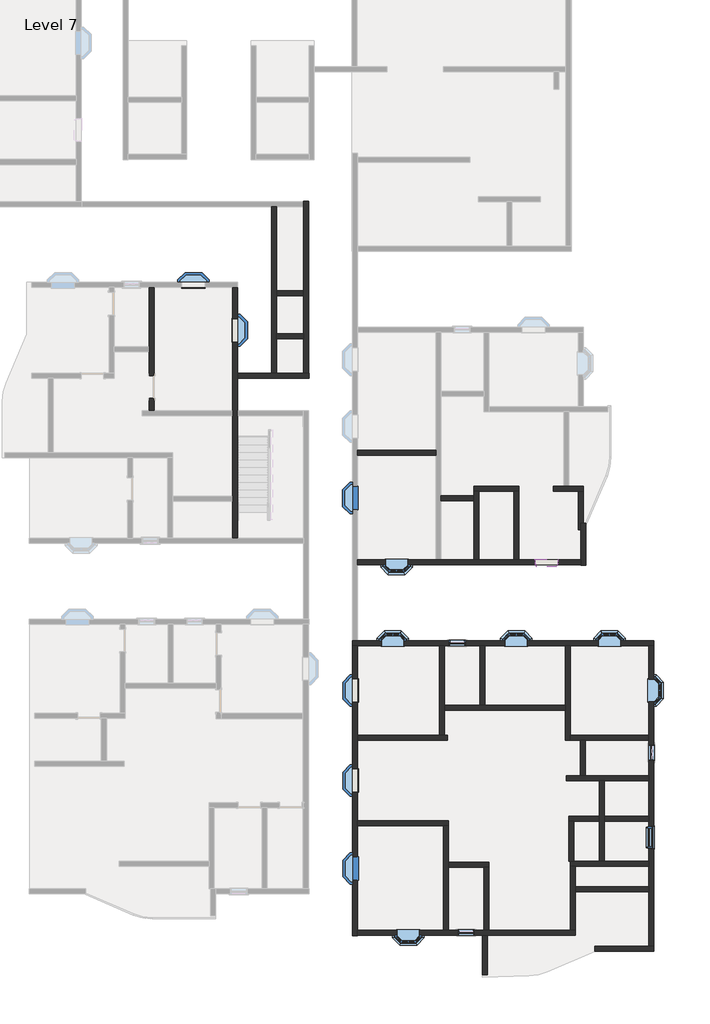
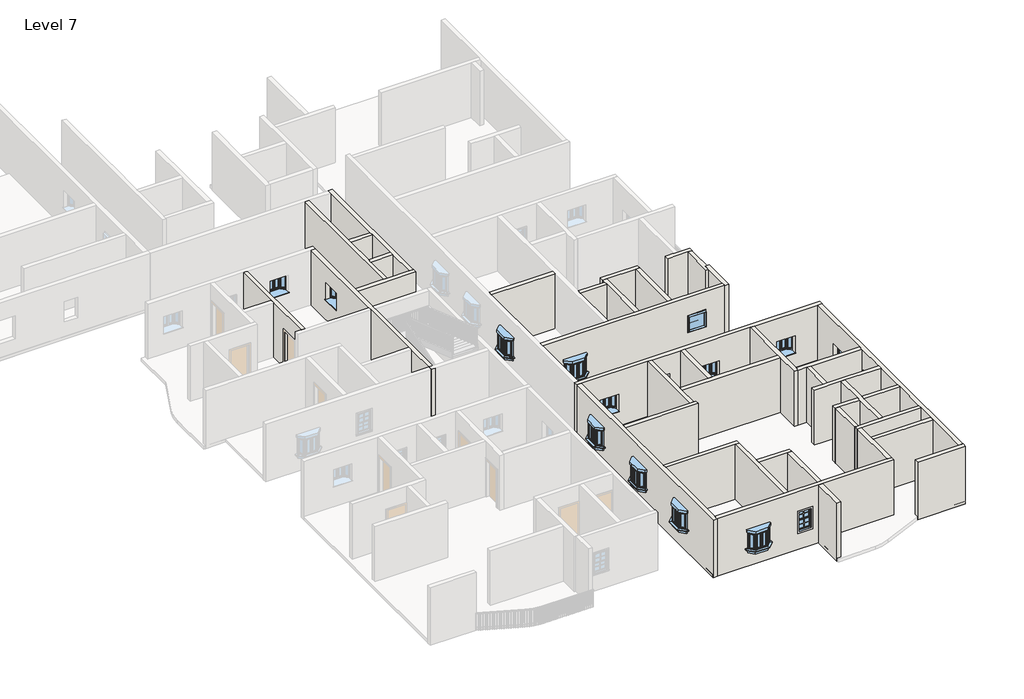
# One storey, part 2 of 14: 40 walls, 17 windows.
"""IFC4 building model written with IfcOpenShell, lengths in millimetres."""

from ifc_helpers import new_model, si_unit, frame, origin, place, context, project, spatial, polyline, outline, extrude, faceted_brep, transform, mapped, element, save
from components import window_910x910mm_67ef725a, window_8debb0fa, windows_sgl_w_glazing_bars_910x910mm_256712d0

model = new_model("IFC4")

# Units and contexts
model_context = context("Model", 3, world=origin())
ifc_project = project(units=[si_unit("LENGTHUNIT", "METRE", prefix="MILLI")], contexts=[model_context])

# Site, building, storey
site = spatial("IfcSite", under=ifc_project)
building = spatial("IfcBuilding", under=site)
storey = spatial("IfcBuildingStorey", under=building, Name="Level 7", Elevation=18288.0)

# Walls
placement = place(None, origin())
element("IfcWall", 1, ObjectType="4.5\" p", at=placement, inside=storey, context=model_context, shape_type="SweptSolid", body=[
    extrude(outline(polyline([(6070.4380523, -28382.7374148), (6070.4380523, -26796.6042694), (6273.6380523, -26796.6042694), (6273.6380523, -28382.7374148), (6070.4380523, -28382.7374148)])), frame((0.0, 0.0, 18288.0), z_axis=(0.0, 0.0, 1.0), x_axis=(1.0, 0.0, 0.0)), (0.0, 0.0, 1.0), 3048.0),
])
element("IfcWall", 2, ObjectType="4.5\" p", at=placement, inside=storey, context=model_context, shape_type="Brep", body=[
    faceted_brep([(10639.6896214, -27431.6042694, 18288.0), (13030.0380523, -27431.6042694, 18288.0), (13030.0380523, -27431.6042694, 21336.0), (10639.6896214, -27431.6042694, 21336.0), (10639.6896214, -27228.4042694, 18288.0), (10639.6896214, -27228.4042694, 21336.0), (12814.1380523, -27228.4042694, 21336.0), (13017.3380523, -27228.4042694, 21336.0), (13030.0380523, -27228.4042694, 21336.0), (13030.0380523, -27228.4042694, 18288.0), (13017.3380523, -27228.4042694, 18288.0), (12814.1380523, -27228.4042694, 18288.0)], [[[0, 1, 2, 3]], [[4, 5, 6, 7, 8, 9, 10, 11]], [[1, 0, 4, 11, 10, 9]], [[2, 1, 9, 8]], [[3, 2, 8, 7, 6, 5]], [[0, 3, 5, 4]]]),
])
element("IfcWall", 3, ObjectType="4.5\" p", at=placement, inside=storey, context=model_context, shape_type="Brep", body=[
    faceted_brep([(1015.8380523, -18878.1542694, 18288.0), (4648.0380523, -18878.1542694, 18288.0), (4648.0380523, -18878.1542694, 21336.0), (1015.8380523, -18878.1542694, 21336.0), (1015.8380523, -18674.9542694, 18288.0), (1015.8380523, -18674.9542694, 21336.0), (4336.8880523, -18674.9542694, 21336.0), (4540.0880523, -18674.9542694, 21336.0), (4648.0380523, -18674.9542694, 21336.0), (4648.0380523, -18674.9542694, 18288.0), (4540.0880523, -18674.9542694, 18288.0), (4336.8880523, -18674.9542694, 18288.0)], [[[0, 1, 2, 3]], [[4, 5, 6, 7, 8, 9, 10, 11]], [[1, 0, 4, 11, 10, 9]], [[2, 1, 9, 8]], [[3, 2, 8, 7, 6, 5]], [[0, 3, 5, 4]]]),
])
element("IfcWall", 4, ObjectType="4.5\" p", at=placement, inside=storey, context=model_context, shape_type="Brep", body=[
    faceted_brep([(4336.8880523, -15049.1042694, 18288.0), (4336.8880523, -18674.9542694, 18288.0), (4336.8880523, -18674.9542694, 21336.0), (4336.8880523, -15049.1042694, 21336.0), (4540.0880523, -15049.1042694, 18288.0), (4540.0880523, -15049.1042694, 21336.0), (4540.0880523, -17455.7542694, 21336.0), (4540.0880523, -17658.9542694, 21336.0), (4540.0880523, -18674.9542694, 21336.0), (4540.0880523, -18674.9542694, 18288.0), (4540.0880523, -17658.9542694, 18288.0), (4540.0880523, -17455.7542694, 18288.0)], [[[0, 1, 2, 3]], [[4, 5, 6, 7, 8, 9, 10, 11]], [[1, 0, 4, 11, 10, 9]], [[3, 2, 8, 7, 6, 5]], [[0, 3, 5, 4]], [[2, 1, 9, 8]]]),
])
element("IfcWall", 5, ObjectType="4.5\" p", at=placement, inside=storey, context=model_context, shape_type="Brep", body=[
    faceted_brep([(4540.0880523, -17658.9542694, 18288.0), (9442.2880523, -17658.9542694, 18288.0), (9442.2880523, -17658.9542694, 21336.0), (4540.0880523, -17658.9542694, 21336.0), (4540.0880523, -17455.7542694, 18288.0), (4540.0880523, -17455.7542694, 21336.0), (5975.1880523, -17455.7542694, 21336.0), (6178.3880523, -17455.7542694, 21336.0), (9442.2880523, -17455.7542694, 21336.0), (9442.2880523, -17455.7542694, 18288.0), (6178.3880523, -17455.7542694, 18288.0), (5975.1880523, -17455.7542694, 18288.0)], [[[0, 1, 2, 3]], [[4, 5, 6, 7, 8, 9, 10, 11]], [[1, 0, 4, 11, 10, 9]], [[3, 2, 8, 7, 6, 5]], [[0, 3, 5, 4]], [[2, 1, 9, 8]]]),
])
element("IfcWall", 6, ObjectType="4.5\" p", at=placement, inside=storey, context=model_context, shape_type="SweptSolid", body=[
    extrude(outline(polyline([(5975.1880523, -17455.7542694), (5975.1880523, -15049.1042694), (6178.3880523, -15049.1042694), (6178.3880523, -17455.7542694), (5975.1880523, -17455.7542694)])), frame((0.0, 0.0, 18288.0), z_axis=(0.0, 0.0, 1.0), x_axis=(1.0, 0.0, 0.0)), (0.0, 0.0, 1.0), 3048.0),
])
element("IfcWall", 7, ObjectType="4.5\" p", at=placement, inside=storey, context=model_context, shape_type="Brep", body=[
    faceted_brep([(9442.2880523, -15049.1042694, 18288.0), (9442.2880523, -17455.7542694, 18288.0), (9442.2880523, -17658.9542694, 18288.0), (9442.2880523, -18871.8042694, 18288.0), (9442.2880523, -18871.8042694, 21336.0), (9442.2880523, -17658.9542694, 21336.0), (9442.2880523, -17455.7542694, 21336.0), (9442.2880523, -15049.1042694, 21336.0), (9645.4880523, -15049.1042694, 18288.0), (9645.4880523, -15049.1042694, 21336.0), (9645.4880523, -18668.6042694, 21336.0), (9645.4880523, -18871.8042694, 21336.0), (9645.4880523, -18871.8042694, 18288.0), (9645.4880523, -18668.6042694, 18288.0)], [[[0, 1, 2, 3, 4, 5, 6, 7]], [[8, 9, 10, 11, 12, 13]], [[3, 2, 1, 0, 8, 13, 12]], [[7, 6, 5, 4, 11, 10, 9]], [[0, 7, 9, 8]], [[4, 3, 12, 11]]]),
])
element("IfcWall", 8, ObjectType="4.5\" p", at=placement, inside=storey, context=model_context, shape_type="Brep", body=[
    faceted_brep([(1015.8380523, -22345.2542694, 18288.0), (4489.2880523, -22345.2542694, 18288.0), (4692.4880523, -22345.2542694, 18288.0), (4692.4880523, -22345.2542694, 21336.0), (4489.2880523, -22345.2542694, 21336.0), (1015.8380523, -22345.2542694, 21336.0), (1015.8380523, -22142.0542694, 18288.0), (1015.8380523, -22142.0542694, 21336.0), (4692.4880523, -22142.0542694, 21336.0), (4692.4880523, -22142.0542694, 18288.0)], [[[0, 1, 2, 3, 4, 5]], [[6, 7, 8, 9]], [[2, 1, 0, 6, 9]], [[5, 4, 3, 8, 7]], [[0, 5, 7, 6]], [[3, 2, 9, 8]]]),
])
element("IfcWall", 9, ObjectType="4.5\" p", at=placement, inside=storey, context=model_context, shape_type="Brep", body=[
    faceted_brep([(4489.2880523, -22345.2542694, 18288.0), (4489.2880523, -26580.7042694, 18288.0), (4489.2880523, -26580.7042694, 21336.0), (4489.2880523, -22345.2542694, 21336.0), (4692.4880523, -22345.2542694, 18288.0), (4692.4880523, -22345.2542694, 21336.0), (4692.4880523, -23818.4542694, 21336.0), (4692.4880523, -24021.6542694, 21336.0), (4692.4880523, -26580.7042694, 21336.0), (4692.4880523, -26580.7042694, 18288.0), (4692.4880523, -24021.6542694, 18288.0), (4692.4880523, -23818.4542694, 18288.0)], [[[0, 1, 2, 3]], [[4, 5, 6, 7, 8, 9, 10, 11]], [[1, 0, 4, 11, 10, 9]], [[3, 2, 8, 7, 6, 5]], [[0, 3, 5, 4]], [[2, 1, 9, 8]]]),
])
element("IfcWall", 10, ObjectType="4.5\" p", at=placement, inside=storey, context=model_context, shape_type="Brep", body=[
    faceted_brep([(4692.4880523, -24021.6542694, 18288.0), (6127.5880523, -24021.6542694, 18288.0), (6330.7880523, -24021.6542694, 18288.0), (6330.7880523, -24021.6542694, 21336.0), (6127.5880523, -24021.6542694, 21336.0), (4692.4880523, -24021.6542694, 21336.0), (4692.4880523, -23818.4542694, 18288.0), (4692.4880523, -23818.4542694, 21336.0), (6330.7880523, -23818.4542694, 21336.0), (6330.7880523, -23818.4542694, 18288.0)], [[[0, 1, 2, 3, 4, 5]], [[6, 7, 8, 9]], [[2, 1, 0, 6, 9]], [[5, 4, 3, 8, 7]], [[0, 5, 7, 6]], [[3, 2, 9, 8]]]),
])
element("IfcWall", 11, ObjectType="4.5\" p", at=placement, inside=storey, context=model_context, shape_type="SweptSolid", body=[
    extrude(outline(polyline([(6127.5880523, -26580.7042694), (6127.5880523, -24021.6542694), (6330.7880523, -24021.6542694), (6330.7880523, -26580.7042694), (6127.5880523, -26580.7042694)])), frame((0.0, 0.0, 18288.0), z_axis=(0.0, 0.0, 1.0), x_axis=(1.0, 0.0, 0.0)), (0.0, 0.0, 1.0), 3048.0),
])
element("IfcWall", 12, ObjectType="4.5\" p", at=placement, inside=storey, context=model_context, shape_type="Brep", body=[
    faceted_brep([(9645.4880523, -18871.8042694, 18288.0), (10051.8880523, -18871.8042694, 18288.0), (10255.0880523, -18871.8042694, 18288.0), (12814.1380523, -18871.8042694, 18288.0), (12814.1380523, -18871.8042694, 21336.0), (10255.0880523, -18871.8042694, 21336.0), (10051.8880523, -18871.8042694, 21336.0), (9645.4880523, -18871.8042694, 21336.0), (9645.4880523, -18668.6042694, 18288.0), (9645.4880523, -18668.6042694, 21336.0), (12814.1380523, -18668.6042694, 21336.0), (12814.1380523, -18668.6042694, 18288.0)], [[[0, 1, 2, 3, 4, 5, 6, 7]], [[8, 9, 10, 11]], [[3, 2, 1, 0, 8, 11]], [[7, 6, 5, 4, 10, 9]], [[0, 7, 9, 8]], [[4, 3, 11, 10]]]),
])
element("IfcWall", 13, ObjectType="4.5\" p", at=placement, inside=storey, context=model_context, shape_type="SweptSolid", body=[
    extrude(outline(polyline([(10051.8880523, -20313.2542694), (10051.8880523, -18871.8042694), (10255.0880523, -18871.8042694), (10255.0880523, -20313.2542694), (10051.8880523, -20313.2542694)])), frame((0.0, 0.0, 18288.0), z_axis=(0.0, 0.0, 1.0), x_axis=(1.0, 0.0, 0.0)), (0.0, 0.0, 1.0), 3048.0),
])
element("IfcWall", 14, ObjectType="4.5\" p", at=placement, inside=storey, context=model_context, shape_type="Brep", body=[
    faceted_brep([(12814.1380523, -20313.2542694, 18288.0), (10255.0880523, -20313.2542694, 18288.0), (10051.8880523, -20313.2542694, 18288.0), (9486.7380523, -20313.2542694, 18288.0), (9486.7380523, -20313.2542694, 21336.0), (10051.8880523, -20313.2542694, 21336.0), (10255.0880523, -20313.2542694, 21336.0), (12814.1380523, -20313.2542694, 21336.0), (12814.1380523, -20516.4542694, 18288.0), (12814.1380523, -20516.4542694, 21336.0), (11017.0880523, -20516.4542694, 21336.0), (10813.8880523, -20516.4542694, 21336.0), (9486.7380523, -20516.4542694, 21336.0), (9486.7380523, -20516.4542694, 18288.0), (10813.8880523, -20516.4542694, 18288.0), (11017.0880523, -20516.4542694, 18288.0)], [[[0, 1, 2, 3, 4, 5, 6, 7]], [[8, 9, 10, 11, 12, 13, 14, 15]], [[3, 2, 1, 0, 8, 15, 14, 13]], [[4, 3, 13, 12]], [[7, 6, 5, 4, 12, 11, 10, 9]], [[0, 7, 9, 8]]]),
])
element("IfcWall", 15, ObjectType="4.5\" p", at=placement, inside=storey, context=model_context, shape_type="Brep", body=[
    faceted_brep([(10813.8880523, -20516.4542694, 18288.0), (10813.8880523, -21951.5542694, 18288.0), (10813.8880523, -22154.7542694, 18288.0), (10813.8880523, -23779.5416506, 18288.0), (10813.8880523, -23779.5416506, 21336.0), (10813.8880523, -22154.7542694, 21336.0), (10813.8880523, -21951.5542694, 21336.0), (10813.8880523, -20516.4542694, 21336.0), (11017.0880523, -20516.4542694, 18288.0), (11017.0880523, -20516.4542694, 21336.0), (11017.0880523, -21951.5542694, 21336.0), (11017.0880523, -22154.7542694, 21336.0), (11017.0880523, -23779.5416506, 21336.0), (11017.0880523, -23779.5416506, 18288.0), (11017.0880523, -22154.7542694, 18288.0), (11017.0880523, -21951.5542694, 18288.0)], [[[0, 1, 2, 3, 4, 5, 6, 7]], [[8, 9, 10, 11, 12, 13, 14, 15]], [[3, 2, 1, 0, 8, 15, 14, 13]], [[7, 6, 5, 4, 12, 11, 10, 9]], [[0, 7, 9, 8]], [[4, 3, 13, 12]]]),
])
element("IfcWall", 16, ObjectType="4.5\" p", at=placement, inside=storey, context=model_context, shape_type="Brep", body=[
    faceted_brep([(12814.1380523, -23779.5416506, 18288.0), (11017.0880523, -23779.5416506, 18288.0), (10813.8880523, -23779.5416506, 18288.0), (9791.5380523, -23779.5416506, 18288.0), (9632.7880523, -23779.5416506, 18288.0), (9632.7880523, -23779.5416506, 21336.0), (9791.5380523, -23779.5416506, 21336.0), (10813.8880523, -23779.5416506, 21336.0), (11017.0880523, -23779.5416506, 21336.0), (12814.1380523, -23779.5416506, 21336.0), (12814.1380523, -23982.7416506, 18288.0), (12814.1380523, -23982.7416506, 21336.0), (9835.9880523, -23982.7416506, 21336.0), (9632.7880523, -23982.7416506, 21336.0), (9632.7880523, -23982.7416506, 18288.0), (9835.9880523, -23982.7416506, 18288.0)], [[[0, 1, 2, 3, 4, 5, 6, 7, 8, 9]], [[10, 11, 12, 13, 14, 15]], [[4, 3, 2, 1, 0, 10, 15, 14]], [[9, 8, 7, 6, 5, 13, 12, 11]], [[0, 9, 11, 10]], [[5, 4, 14, 13]]]),
])
element("IfcWall", 17, ObjectType="4.5\" p", at=placement, inside=storey, context=model_context, shape_type="Brep", body=[
    faceted_brep([(9632.7880523, -23982.7416506, 18288.0), (9632.7880523, -26580.7042694, 18288.0), (9632.7880523, -26580.7042694, 21336.0), (9632.7880523, -23982.7416506, 21336.0), (9835.9880523, -23982.7416506, 18288.0), (9835.9880523, -23982.7416506, 21336.0), (9835.9880523, -24805.3496998, 21336.0), (9835.9880523, -25008.5496998, 21336.0), (9835.9880523, -26580.7042694, 21336.0), (9835.9880523, -26580.7042694, 18288.0), (9835.9880523, -25008.5496998, 18288.0), (9835.9880523, -24805.3496998, 18288.0)], [[[0, 1, 2, 3]], [[4, 5, 6, 7, 8, 9, 10, 11]], [[1, 0, 4, 11, 10, 9]], [[3, 2, 8, 7, 6, 5]], [[2, 1, 9, 8]], [[0, 3, 5, 4]]]),
])
element("IfcWall", 18, ObjectType="4.5\" p", at=placement, inside=storey, context=model_context, shape_type="SweptSolid", body=[
    extrude(outline(polyline([(12814.1380523, -25008.5496998), (9835.9880523, -25008.5496998), (9835.9880523, -24805.3496998), (12814.1380523, -24805.3496998), (12814.1380523, -25008.5496998)])), frame((0.0, 0.0, 18288.0), z_axis=(0.0, 0.0, 1.0), x_axis=(1.0, 0.0, 0.0)), (0.0, 0.0, 1.0), 3048.0),
])
element("IfcWall", 19, ObjectType="4.5\" p", at=placement, inside=storey, context=model_context, shape_type="Brep", body=[
    faceted_brep([(-7432.737215, -5015.2916506, 20421.6), (-7432.737215, -5015.2916506, 18288.0), (-7432.737215, -5523.2916506, 18288.0), (-7432.737215, -5523.2916506, 21336.0), (-7432.737215, -3135.6916506, 21336.0), (-7432.737215, -2932.4916506, 21336.0), (-7432.737215, -525.8416506, 21336.0), (-7432.737215, -525.8416506, 18288.0), (-7432.737215, -2932.4916506, 18288.0), (-7432.737215, -3135.6916506, 18288.0), (-7432.737215, -4100.8916506, 18288.0), (-7432.737215, -4100.8916506, 20421.6), (-7229.537215, -5523.2916506, 18288.0), (-7229.537215, -5015.2916506, 18288.0), (-7229.537215, -5015.2916506, 20421.6), (-7229.537215, -4100.8916506, 20421.6), (-7229.537215, -4100.8916506, 18288.0), (-7229.537215, -525.8416506, 18288.0), (-7229.537215, -525.8416506, 21336.0), (-7229.537215, -5523.2916506, 21336.0)], [[[0, 1, 2, 3, 4, 5, 6, 7, 8, 9, 10, 11]], [[12, 13, 14, 15, 16, 17, 18, 19]], [[2, 1, 13, 12]], [[10, 9, 8, 7, 17, 16]], [[6, 5, 4, 3, 19, 18]], [[7, 6, 18, 17]], [[3, 2, 12, 19]], [[14, 13, 1, 0]], [[15, 14, 0, 11]], [[16, 15, 11, 10]]]),
])
element("IfcWall", 20, ObjectType="4.5\" p", at=placement, inside=storey, context=model_context, shape_type="Brep", body=[
    faceted_brep([(-3857.687215, -4202.4916506, 18288.0), (-961.4891351, -4202.4916506, 18288.0), (-961.4891351, -4202.4916506, 21336.0), (-3857.687215, -4202.4916506, 21336.0), (-3857.687215, -3999.2916506, 18288.0), (-3857.687215, -3999.2916506, 21336.0), (-2472.7891351, -3999.2916506, 21336.0), (-2269.5891351, -3999.2916506, 21336.0), (-1177.3891351, -3999.2916506, 21336.0), (-974.1891351, -3999.2916506, 21336.0), (-961.4891351, -3999.2916506, 21336.0), (-961.4891351, -3999.2916506, 18288.0), (-974.1891351, -3999.2916506, 18288.0), (-1177.3891351, -3999.2916506, 18288.0), (-2269.5891351, -3999.2916506, 18288.0), (-2472.7891351, -3999.2916506, 18288.0)], [[[0, 1, 2, 3]], [[4, 5, 6, 7, 8, 9, 10, 11, 12, 13, 14, 15]], [[1, 0, 4, 15, 14, 13, 12, 11]], [[2, 1, 11, 10]], [[3, 2, 10, 9, 8, 7, 6, 5]], [[0, 3, 5, 4]]]),
])
element("IfcWall", 21, ObjectType="4.5\" p", at=placement, inside=storey, context=model_context, shape_type="SweptSolid", body=[
    extrude(outline(polyline([(-1177.3891351, -868.7416506), (-2269.5891351, -868.7416506), (-2269.5891351, -665.5416506), (-1177.3891351, -665.5416506), (-1177.3891351, -868.7416506)])), frame((0.0, 0.0, 18288.0), z_axis=(0.0, 0.0, 1.0), x_axis=(1.0, 0.0, 0.0)), (0.0, 0.0, 1.0), 3048.0),
])
element("IfcWall", 22, ObjectType="4.5\" p", at=placement, inside=storey, context=model_context, shape_type="SweptSolid", body=[
    extrude(outline(polyline([(-1177.3891351, -2597.8466506), (-2269.5891351, -2597.8466506), (-2269.5891351, -2394.6466506), (-1177.3891351, -2394.6466506), (-1177.3891351, -2597.8466506)])), frame((0.0, 0.0, 18288.0), z_axis=(0.0, 0.0, 1.0), x_axis=(1.0, 0.0, 0.0)), (0.0, 0.0, 1.0), 3048.0),
])
element("IfcWall", 23, ObjectType="4.5\" p", at=placement, inside=storey, context=model_context, shape_type="SweptSolid", body=[
    extrude(outline(polyline([(5721.1880523, -9162.6542694), (4387.6880523, -9162.6542694), (4387.6880523, -8959.4542694), (5721.1880523, -8959.4542694), (5721.1880523, -9162.6542694)])), frame((0.0, 0.0, 18288.0), z_axis=(0.0, 0.0, 1.0), x_axis=(1.0, 0.0, 0.0)), (0.0, 0.0, 1.0), 3048.0),
])
element("IfcWall", 24, ObjectType="4.5\" p", at=placement, inside=storey, context=model_context, shape_type="Brep", body=[
    faceted_brep([(5721.1880523, -8781.6542694, 18288.0), (5924.3880523, -8781.6542694, 18288.0), (7359.4880523, -8781.6542694, 18288.0), (7562.6880523, -8781.6542694, 18288.0), (7562.6880523, -8781.6542694, 21336.0), (7359.4880523, -8781.6542694, 21336.0), (5924.3880523, -8781.6542694, 21336.0), (5721.1880523, -8781.6542694, 21336.0), (5721.1880523, -8578.4542694, 18288.0), (5721.1880523, -8578.4542694, 21336.0), (7562.6880523, -8578.4542694, 21336.0), (7562.6880523, -8578.4542694, 18288.0)], [[[0, 1, 2, 3, 4, 5, 6, 7]], [[8, 9, 10, 11]], [[3, 2, 1, 0, 8, 11]], [[7, 6, 5, 4, 10, 9]], [[0, 7, 9, 8]], [[4, 3, 11, 10]]]),
])
element("IfcWall", 25, ObjectType="4.5\" p", at=placement, inside=storey, context=model_context, shape_type="Brep", body=[
    faceted_brep([(5721.1880523, -8781.6542694, 18288.0), (5721.1880523, -8959.4542694, 18288.0), (5721.1880523, -9162.6542694, 18288.0), (5721.1880523, -11556.6042694, 18288.0), (5721.1880523, -11556.6042694, 21336.0), (5721.1880523, -9162.6542694, 21336.0), (5721.1880523, -8959.4542694, 21336.0), (5721.1880523, -8781.6542694, 21336.0), (5924.3880523, -8781.6542694, 18288.0), (5924.3880523, -8781.6542694, 21336.0), (5924.3880523, -11556.6042694, 21336.0), (5924.3880523, -11556.6042694, 18288.0)], [[[0, 1, 2, 3, 4, 5, 6, 7]], [[8, 9, 10, 11]], [[3, 2, 1, 0, 8, 11]], [[7, 6, 5, 4, 10, 9]], [[0, 7, 9, 8]], [[4, 3, 11, 10]]]),
])
element("IfcWall", 26, ObjectType="4.5\" p", at=placement, inside=storey, context=model_context, shape_type="SweptSolid", body=[
    extrude(outline(polyline([(7359.4880523, -11556.6042694), (7359.4880523, -8781.6542694), (7562.6880523, -8781.6542694), (7562.6880523, -11556.6042694), (7359.4880523, -11556.6042694)])), frame((0.0, 0.0, 18288.0), z_axis=(0.0, 0.0, 1.0), x_axis=(1.0, 0.0, 0.0)), (0.0, 0.0, 1.0), 3048.0),
])
element("IfcWall", 27, ObjectType="4.5\" p", at=placement, inside=storey, context=model_context, shape_type="SweptSolid", body=[
    extrude(outline(polyline([(4184.4880523, -7333.8542694), (1007.0108649, -7333.8542694), (1007.0108649, -7130.6542694), (4184.4880523, -7130.6542694), (4184.4880523, -7333.8542694)])), frame((0.0, 0.0, 18288.0), z_axis=(0.0, 0.0, 1.0), x_axis=(1.0, 0.0, 0.0)), (0.0, 0.0, 1.0), 3048.0),
])
element("IfcWall", 28, ObjectType="4.5\" p", at=placement, inside=storey, context=model_context, shape_type="Brep", body=[
    faceted_brep([(8953.3380523, -8781.6542694, 18288.0), (9956.6380523, -8781.6542694, 18288.0), (10159.8380523, -8781.6542694, 18288.0), (10172.5380523, -8781.6542694, 18288.0), (10172.5380523, -8781.6542694, 21336.0), (10159.8380523, -8781.6542694, 21336.0), (9956.6380523, -8781.6542694, 21336.0), (8953.3380523, -8781.6542694, 21336.0), (8953.3380523, -8578.4542694, 18288.0), (8953.3380523, -8578.4542694, 21336.0), (9371.2322031, -8578.4542694, 21336.0), (9574.4322031, -8578.4542694, 21336.0), (10172.5380523, -8578.4542694, 21336.0), (10172.5380523, -8578.4542694, 18288.0), (9574.4322031, -8578.4542694, 18288.0), (9371.2322031, -8578.4542694, 18288.0)], [[[0, 1, 2, 3, 4, 5, 6, 7]], [[8, 9, 10, 11, 12, 13, 14, 15]], [[3, 2, 1, 0, 8, 15, 14, 13]], [[4, 3, 13, 12]], [[7, 6, 5, 4, 12, 11, 10, 9]], [[0, 7, 9, 8]]]),
])
element("IfcWall", 29, ObjectType="4.5\" p", at=placement, inside=storey, context=model_context, shape_type="SweptSolid", body=[
    extrude(outline(polyline([(9956.6380523, -10352.8912671), (9956.6380523, -8781.6542694), (10159.8380523, -8781.6542694), (10159.8380523, -10352.8912671), (9956.6380523, -10352.8912671)])), frame((0.0, 0.0, 18288.0), z_axis=(0.0, 0.0, 1.0), x_axis=(1.0, 0.0, 0.0)), (0.0, 0.0, 1.0), 3048.0),
])
element("IfcWall", 30, ObjectType="4.5\" p", at=placement, inside=storey, context=model_context, shape_type="Brep", body=[
    faceted_brep([(12814.1380523, -21951.5542694, 21336.0), (12814.1380523, -21951.5542694, 18288.0), (11017.0880523, -21951.5542694, 18288.0), (11017.0880523, -21951.5542694, 21336.0), (12814.1380523, -22154.7542694, 18288.0), (12814.1380523, -22154.7542694, 21336.0), (11017.0880523, -22154.7542694, 21336.0), (11017.0880523, -22154.7542694, 18288.0)], [[[0, 1, 2, 3]], [[4, 5, 6, 7]], [[1, 4, 7, 2]], [[5, 0, 3, 6]], [[1, 0, 5, 4]], [[3, 2, 7, 6]]]),
    faceted_brep([(9588.3380523, -21951.5542694, 18288.0), (9588.3380523, -21951.5542694, 21336.0), (10813.8880523, -21951.5542694, 21336.0), (10813.8880523, -21951.5542694, 18288.0), (9588.3380523, -22154.7542694, 21336.0), (9588.3380523, -22154.7542694, 18288.0), (9791.5380523, -22154.7542694, 18288.0), (10813.8880523, -22154.7542694, 18288.0), (10813.8880523, -22154.7542694, 21336.0), (9791.5380523, -22154.7542694, 21336.0)], [[[0, 1, 2, 3]], [[4, 5, 6, 7, 8, 9]], [[5, 0, 3, 7, 6]], [[1, 4, 9, 8, 2]], [[3, 2, 8, 7]], [[1, 0, 5, 4]]]),
])
element("IfcWall", 31, ObjectType="4.5\" p", at=placement, inside=storey, context=model_context, shape_type="Brep", body=[
    faceted_brep([(9588.3380523, -22154.7542694, 18288.0), (9588.3380523, -23779.5416506, 18288.0), (9588.3380523, -23779.5416506, 21336.0), (9588.3380523, -22154.7542694, 21336.0), (9791.5380523, -22154.7542694, 18288.0), (9791.5380523, -22154.7542694, 21336.0), (9791.5380523, -23779.5416506, 21336.0), (9791.5380523, -23779.5416506, 18288.0), (9632.7880523, -23779.5416506, 18288.0), (9632.7880523, -23779.5416506, 21336.0)], [[[0, 1, 2, 3]], [[4, 5, 6, 7]], [[1, 0, 4, 7, 8]], [[3, 2, 9, 6, 5]], [[2, 1, 8, 7, 6, 9]], [[0, 3, 5, 4]]]),
])
element("IfcWall", 32, ObjectType="9\"", at=placement, inside=storey, context=model_context, shape_type="Brep", body=[
    faceted_brep([(799.9380523, -15049.1042694, 18288.0), (812.6380523, -15049.1042694, 18288.0), (1015.8380523, -15049.1042694, 18288.0), (4336.8880523, -15049.1042694, 18288.0), (4540.0880523, -15049.1042694, 18288.0), (5975.1880523, -15049.1042694, 18288.0), (6178.3880523, -15049.1042694, 18288.0), (9442.2880523, -15049.1042694, 18288.0), (9645.4880523, -15049.1042694, 18288.0), (12814.1380523, -15049.1042694, 18288.0), (13017.3380523, -15049.1042694, 18288.0), (13030.0380523, -15049.1042694, 18288.0), (13030.0380523, -15049.1042694, 21336.0), (13017.3380523, -15049.1042694, 21336.0), (12814.1380523, -15049.1042694, 21336.0), (9645.4880523, -15049.1042694, 21336.0), (9442.2880523, -15049.1042694, 21336.0), (6178.3880523, -15049.1042694, 21336.0), (5975.1880523, -15049.1042694, 21336.0), (4540.0880523, -15049.1042694, 21336.0), (4336.8880523, -15049.1042694, 21336.0), (1015.8380523, -15049.1042694, 21336.0), (812.6380523, -15049.1042694, 21336.0), (799.9380523, -15049.1042694, 21336.0), (1983.2380523, -15049.1042694, 20112.4), (2893.2380523, -15049.1042694, 20112.4), (2893.2380523, -15049.1042694, 19202.4), (1983.2380523, -15049.1042694, 19202.4), (10774.8130523, -15049.1042694, 20112.4), (11684.8130523, -15049.1042694, 20112.4), (11684.8130523, -15049.1042694, 19202.4), (10774.8130523, -15049.1042694, 19202.4), (6993.3880523, -15049.1042694, 20112.4), (7903.3880523, -15049.1042694, 20112.4), (7903.3880523, -15049.1042694, 19202.4), (6993.3880523, -15049.1042694, 19202.4), (4717.8880523, -15049.1042694, 20269.2), (5378.2880523, -15049.1042694, 20269.2), (5378.2880523, -15049.1042694, 19202.4), (4717.8880523, -15049.1042694, 19202.4), (799.9380523, -14845.9042694, 18288.0), (799.9380523, -14845.9042694, 21336.0), (803.8108649, -14845.9042694, 21336.0), (1007.0108649, -14845.9042694, 21336.0), (13030.0380523, -14845.9042694, 21336.0), (13030.0380523, -14845.9042694, 18288.0), (1007.0108649, -14845.9042694, 18288.0), (803.8108649, -14845.9042694, 18288.0), (1983.2380523, -14845.9042694, 20112.4), (1983.2380523, -14845.9042694, 19202.4), (2893.2380523, -14845.9042694, 19202.4), (2893.2380523, -14845.9042694, 20112.4), (10774.8130523, -14845.9042694, 20112.4), (10774.8130523, -14845.9042694, 19202.4), (11684.8130523, -14845.9042694, 19202.4), (11684.8130523, -14845.9042694, 20112.4), (6993.3880523, -14845.9042694, 20112.4), (6993.3880523, -14845.9042694, 19202.4), (7903.3880523, -14845.9042694, 19202.4), (7903.3880523, -14845.9042694, 20112.4), (4717.8880523, -14845.9042694, 20269.2), (4717.8880523, -14845.9042694, 19202.4), (5378.2880523, -14845.9042694, 19202.4), (5378.2880523, -14845.9042694, 20269.2)], [[[0, 1, 2, 3, 4, 5, 6, 7, 8, 9, 10, 11, 12, 13, 14, 15, 16, 17, 18, 19, 20, 21, 22, 23], [24, 25, 26, 27], [28, 29, 30, 31], [32, 33, 34, 35], [36, 37, 38, 39]], [[40, 41, 42, 43, 44, 45, 46, 47], [48, 49, 50, 51], [52, 53, 54, 55], [56, 57, 58, 59], [60, 61, 62, 63]], [[11, 10, 9, 8, 7, 6, 5, 4, 3, 2, 1, 0, 40, 47, 46, 45]], [[12, 11, 45, 44]], [[23, 22, 21, 20, 19, 18, 17, 16, 15, 14, 13, 12, 44, 43, 42, 41]], [[0, 23, 41, 40]], [[49, 48, 24, 27]], [[50, 49, 27, 26]], [[51, 50, 26, 25]], [[48, 51, 25, 24]], [[53, 52, 28, 31]], [[54, 53, 31, 30]], [[55, 54, 30, 29]], [[52, 55, 29, 28]], [[57, 56, 32, 35]], [[58, 57, 35, 34]], [[59, 58, 34, 33]], [[56, 59, 33, 32]], [[61, 60, 36, 39]], [[62, 61, 39, 38]], [[63, 62, 38, 37]], [[60, 63, 37, 36]]]),
])
element("IfcWall", 33, ObjectType="9\"", at=placement, inside=storey, context=model_context, shape_type="Brep", body=[
    faceted_brep([(12814.1380523, -15049.1042694, 18288.0), (12814.1380523, -18668.6042694, 18288.0), (12814.1380523, -18871.8042694, 18288.0), (12814.1380523, -20313.2542694, 18288.0), (12814.1380523, -20516.4542694, 18288.0), (12814.1380523, -21951.5542694, 18288.0), (12814.1380523, -22154.7542694, 18288.0), (12814.1380523, -23779.5416506, 18288.0), (12814.1380523, -23982.7416506, 18288.0), (12814.1380523, -24805.3496998, 18288.0), (12814.1380523, -25008.5496998, 18288.0), (12814.1380523, -27228.4042694, 18288.0), (12814.1380523, -27228.4042694, 21336.0), (12814.1380523, -25008.5496998, 21336.0), (12814.1380523, -24805.3496998, 21336.0), (12814.1380523, -23982.7416506, 21336.0), (12814.1380523, -23779.5416506, 21336.0), (12814.1380523, -22154.7542694, 21336.0), (12814.1380523, -21951.5542694, 21336.0), (12814.1380523, -20516.4542694, 21336.0), (12814.1380523, -20313.2542694, 21336.0), (12814.1380523, -18871.8042694, 21336.0), (12814.1380523, -18668.6042694, 21336.0), (12814.1380523, -15049.1042694, 21336.0), (12814.1380523, -16403.8542694, 20112.4), (12814.1380523, -17313.8542694, 20112.4), (12814.1380523, -17313.8542694, 19202.4), (12814.1380523, -16403.8542694, 19202.4), (12814.1380523, -23270.1542694, 20112.4), (12814.1380523, -23270.1542694, 19202.4), (12814.1380523, -22360.1542694, 19202.4), (12814.1380523, -22360.1542694, 20112.4), (12814.1380523, -19049.6042694, 20269.2), (12814.1380523, -19710.0042694, 20269.2), (12814.1380523, -19710.0042694, 19202.4), (12814.1380523, -19049.6042694, 19202.4), (13017.3380523, -15049.1042694, 18288.0), (13017.3380523, -15049.1042694, 21336.0), (13017.3380523, -27228.4042694, 21336.0), (13017.3380523, -27228.4042694, 18288.0), (13017.3380523, -16403.8542694, 20112.4), (13017.3380523, -16403.8542694, 19202.4), (13017.3380523, -17313.8542694, 19202.4), (13017.3380523, -17313.8542694, 20112.4), (13017.3380523, -23270.1542694, 20112.4), (13017.3380523, -22360.1542694, 20112.4), (13017.3380523, -22360.1542694, 19202.4), (13017.3380523, -23270.1542694, 19202.4), (13017.3380523, -19049.6042694, 20269.2), (13017.3380523, -19049.6042694, 19202.4), (13017.3380523, -19710.0042694, 19202.4), (13017.3380523, -19710.0042694, 20269.2)], [[[0, 1, 2, 3, 4, 5, 6, 7, 8, 9, 10, 11, 12, 13, 14, 15, 16, 17, 18, 19, 20, 21, 22, 23], [24, 25, 26, 27], [28, 29, 30, 31], [32, 33, 34, 35]], [[36, 37, 38, 39], [40, 41, 42, 43], [44, 45, 46, 47], [48, 49, 50, 51]], [[11, 10, 9, 8, 7, 6, 5, 4, 3, 2, 1, 0, 36, 39]], [[23, 22, 21, 20, 19, 18, 17, 16, 15, 14, 13, 12, 38, 37]], [[0, 23, 37, 36]], [[12, 11, 39, 38]], [[41, 40, 24, 27]], [[42, 41, 27, 26]], [[43, 42, 26, 25]], [[40, 43, 25, 24]], [[29, 28, 44, 47]], [[30, 29, 47, 46]], [[31, 30, 46, 45]], [[28, 31, 45, 44]], [[49, 48, 32, 35]], [[50, 49, 35, 34]], [[51, 50, 34, 33]], [[48, 51, 33, 32]]]),
])
element("IfcWall", 34, ObjectType="9\"", at=placement, inside=storey, context=model_context, shape_type="Brep", body=[
    faceted_brep([(812.6380523, -15049.1042694, 18288.0), (812.6380523, -26796.6042694, 18288.0), (812.6380523, -26796.6042694, 21336.0), (812.6380523, -15049.1042694, 21336.0), (812.6380523, -24527.4542694, 20398.0), (812.6380523, -24527.4542694, 19488.0), (812.6380523, -23617.4542694, 19488.0), (812.6380523, -23617.4542694, 20398.0), (812.6380523, -20965.1042694, 20398.0), (812.6380523, -20965.1042694, 19488.0), (812.6380523, -20055.1042694, 19488.0), (812.6380523, -20055.1042694, 20398.0), (812.6380523, -17317.0292694, 20398.0), (812.6380523, -17317.0292694, 19488.0), (812.6380523, -16407.0292694, 19488.0), (812.6380523, -16407.0292694, 20398.0), (1015.8380523, -15049.1042694, 18288.0), (1015.8380523, -15049.1042694, 21336.0), (1015.8380523, -18674.9542694, 21336.0), (1015.8380523, -18878.1542694, 21336.0), (1015.8380523, -22142.0542694, 21336.0), (1015.8380523, -22345.2542694, 21336.0), (1015.8380523, -26580.7042694, 21336.0), (1015.8380523, -26783.9042694, 21336.0), (1015.8380523, -26796.6042694, 21336.0), (1015.8380523, -26796.6042694, 18288.0), (1015.8380523, -26783.9042694, 18288.0), (1015.8380523, -26580.7042694, 18288.0), (1015.8380523, -22345.2542694, 18288.0), (1015.8380523, -22142.0542694, 18288.0), (1015.8380523, -18878.1542694, 18288.0), (1015.8380523, -18674.9542694, 18288.0), (1015.8380523, -24527.4542694, 20398.0), (1015.8380523, -23617.4542694, 20398.0), (1015.8380523, -23617.4542694, 19488.0), (1015.8380523, -24527.4542694, 19488.0), (1015.8380523, -20965.1042694, 20398.0), (1015.8380523, -20055.1042694, 20398.0), (1015.8380523, -20055.1042694, 19488.0), (1015.8380523, -20965.1042694, 19488.0), (1015.8380523, -17317.0292694, 20398.0), (1015.8380523, -16407.0292694, 20398.0), (1015.8380523, -16407.0292694, 19488.0), (1015.8380523, -17317.0292694, 19488.0)], [[[0, 1, 2, 3], [4, 5, 6, 7], [8, 9, 10, 11], [12, 13, 14, 15]], [[16, 17, 18, 19, 20, 21, 22, 23, 24, 25, 26, 27, 28, 29, 30, 31], [32, 33, 34, 35], [36, 37, 38, 39], [40, 41, 42, 43]], [[1, 0, 16, 31, 30, 29, 28, 27, 26, 25]], [[2, 1, 25, 24]], [[3, 2, 24, 23, 22, 21, 20, 19, 18, 17]], [[0, 3, 17, 16]], [[5, 4, 32, 35]], [[6, 5, 35, 34]], [[7, 6, 34, 33]], [[4, 7, 33, 32]], [[9, 8, 36, 39]], [[10, 9, 39, 38]], [[11, 10, 38, 37]], [[8, 11, 37, 36]], [[13, 12, 40, 43]], [[14, 13, 43, 42]], [[15, 14, 42, 41]], [[12, 15, 41, 40]]]),
])
element("IfcWall", 35, ObjectType="9\"", at=placement, inside=storey, context=model_context, shape_type="Brep", body=[
    faceted_brep([(1015.8380523, -26783.9042694, 18288.0), (9835.9880523, -26783.9042694, 18288.0), (9835.9880523, -26783.9042694, 21336.0), (1015.8380523, -26783.9042694, 21336.0), (3521.8880523, -26783.9042694, 20112.4), (3521.8880523, -26783.9042694, 19202.4), (2611.8880523, -26783.9042694, 19202.4), (2611.8880523, -26783.9042694, 20112.4), (5079.8380523, -26783.9042694, 20269.2), (5740.2380523, -26783.9042694, 20269.2), (5740.2380523, -26783.9042694, 19202.4), (5079.8380523, -26783.9042694, 19202.4), (1015.8380523, -26580.7042694, 18288.0), (1015.8380523, -26580.7042694, 21336.0), (4489.2880523, -26580.7042694, 21336.0), (4692.4880523, -26580.7042694, 21336.0), (6127.5880523, -26580.7042694, 21336.0), (6330.7880523, -26580.7042694, 21336.0), (9632.7880523, -26580.7042694, 21336.0), (9835.9880523, -26580.7042694, 21336.0), (9835.9880523, -26580.7042694, 18288.0), (9632.7880523, -26580.7042694, 18288.0), (6330.7880523, -26580.7042694, 18288.0), (6127.5880523, -26580.7042694, 18288.0), (4692.4880523, -26580.7042694, 18288.0), (4489.2880523, -26580.7042694, 18288.0), (3521.8880523, -26580.7042694, 20112.4), (2611.8880523, -26580.7042694, 20112.4), (2611.8880523, -26580.7042694, 19202.4), (3521.8880523, -26580.7042694, 19202.4), (5079.8380523, -26580.7042694, 20269.2), (5079.8380523, -26580.7042694, 19202.4), (5740.2380523, -26580.7042694, 19202.4), (5740.2380523, -26580.7042694, 20269.2)], [[[0, 1, 2, 3], [4, 5, 6, 7], [8, 9, 10, 11]], [[12, 13, 14, 15, 16, 17, 18, 19, 20, 21, 22, 23, 24, 25], [26, 27, 28, 29], [30, 31, 32, 33]], [[1, 0, 12, 25, 24, 23, 22, 21, 20]], [[3, 2, 19, 18, 17, 16, 15, 14, 13]], [[0, 3, 13, 12]], [[2, 1, 20, 19]], [[5, 4, 26, 29]], [[6, 5, 29, 28]], [[7, 6, 28, 27]], [[4, 7, 27, 26]], [[31, 30, 8, 11]], [[32, 31, 11, 10]], [[33, 32, 10, 9]], [[30, 33, 9, 8]]]),
])
element("IfcWall", 36, ObjectType="9\" w", at=placement, inside=storey, context=model_context, shape_type="Brep", body=[
    faceted_brep([(-4060.887215, -525.8416506, 18288.0), (-4060.887215, -5523.2916506, 18288.0), (-4060.887215, -5726.4916506, 18288.0), (-4060.887215, -8990.3916506, 18288.0), (-4060.887215, -9193.5916506, 18288.0), (-4060.887215, -10901.7416506, 18288.0), (-4060.887215, -10901.7416506, 21336.0), (-4060.887215, -9193.5916506, 21336.0), (-4060.887215, -8990.3916506, 21336.0), (-4060.887215, -5726.4916506, 21336.0), (-4060.887215, -5523.2916506, 21336.0), (-4060.887215, -525.8416506, 21336.0), (-4060.887215, -1807.5666506, 20398.0), (-4060.887215, -2717.5666506, 20398.0), (-4060.887215, -2717.5666506, 19488.0), (-4060.887215, -1807.5666506, 19488.0), (-3857.687215, -525.8416506, 18288.0), (-3857.687215, -525.8416506, 21336.0), (-3857.687215, -3999.2916506, 21336.0), (-3857.687215, -4202.4916506, 21336.0), (-3857.687215, -5523.2916506, 21336.0), (-3857.687215, -5726.4916506, 21336.0), (-3857.687215, -10901.7416506, 21336.0), (-3857.687215, -10901.7416506, 18288.0), (-3857.687215, -5726.4916506, 18288.0), (-3857.687215, -5523.2916506, 18288.0), (-3857.687215, -4202.4916506, 18288.0), (-3857.687215, -3999.2916506, 18288.0), (-3857.687215, -1807.5666506, 20398.0), (-3857.687215, -1807.5666506, 19488.0), (-3857.687215, -2717.5666506, 19488.0), (-3857.687215, -2717.5666506, 20398.0)], [[[0, 1, 2, 3, 4, 5, 6, 7, 8, 9, 10, 11], [12, 13, 14, 15]], [[16, 17, 18, 19, 20, 21, 22, 23, 24, 25, 26, 27], [28, 29, 30, 31]], [[5, 4, 3, 2, 1, 0, 16, 27, 26, 25, 24, 23]], [[6, 5, 23, 22]], [[11, 10, 9, 8, 7, 6, 22, 21, 20, 19, 18, 17]], [[0, 11, 17, 16]], [[29, 28, 12, 15]], [[30, 29, 15, 14]], [[31, 30, 14, 13]], [[28, 31, 13, 12]]]),
])
element("IfcWall", 37, ObjectType="9\" w", at=placement, inside=storey, context=model_context, shape_type="Brep", body=[
    faceted_brep([(-2269.5891351, -3999.2916506, 18288.0), (-2269.5891351, -2597.8466506, 18288.0), (-2269.5891351, -2394.6466506, 18288.0), (-2269.5891351, -868.7416506, 18288.0), (-2269.5891351, -665.5416506, 18288.0), (-2269.5891351, 2750.7583494, 18288.0), (-2269.5891351, 2750.7583494, 21336.0), (-2269.5891351, -665.5416506, 21336.0), (-2269.5891351, -868.7416506, 21336.0), (-2269.5891351, -2394.6466506, 21336.0), (-2269.5891351, -2597.8466506, 21336.0), (-2269.5891351, -3999.2916506, 21336.0), (-2472.7891351, -3999.2916506, 18288.0), (-2472.7891351, -3999.2916506, 21336.0), (-2472.7891351, 2750.7583494, 21336.0), (-2472.7891351, 2750.7583494, 18288.0)], [[[0, 1, 2, 3, 4, 5, 6, 7, 8, 9, 10, 11]], [[12, 13, 14, 15]], [[5, 4, 3, 2, 1, 0, 12, 15]], [[11, 10, 9, 8, 7, 6, 14, 13]], [[0, 11, 13, 12]], [[6, 5, 15, 14]]]),
])
element("IfcWall", 38, ObjectType="9\" w", at=placement, inside=storey, context=model_context, shape_type="Brep", body=[
    faceted_brep([(-974.1891351, -3999.2916506, 18288.0), (-974.1891351, 2966.6583494, 18288.0), (-974.1891351, 2966.6583494, 21336.0), (-974.1891351, -3999.2916506, 21336.0), (-1177.3891351, -3999.2916506, 18288.0), (-1177.3891351, -3999.2916506, 21336.0), (-1177.3891351, -2597.8466506, 21336.0), (-1177.3891351, -2394.6466506, 21336.0), (-1177.3891351, -868.7416506, 21336.0), (-1177.3891351, -665.5416506, 21336.0), (-1177.3891351, 2750.7583494, 21336.0), (-1177.3891351, 2953.9583494, 21336.0), (-1177.3891351, 2966.6583494, 21336.0), (-1177.3891351, 2966.6583494, 18288.0), (-1177.3891351, 2953.9583494, 18288.0), (-1177.3891351, 2750.7583494, 18288.0), (-1177.3891351, -665.5416506, 18288.0), (-1177.3891351, -868.7416506, 18288.0), (-1177.3891351, -2394.6466506, 18288.0), (-1177.3891351, -2597.8466506, 18288.0)], [[[0, 1, 2, 3]], [[4, 5, 6, 7, 8, 9, 10, 11, 12, 13, 14, 15, 16, 17, 18, 19]], [[1, 0, 4, 19, 18, 17, 16, 15, 14, 13]], [[2, 1, 13, 12]], [[3, 2, 12, 11, 10, 9, 8, 7, 6, 5]], [[0, 3, 5, 4]]]),
])
element("IfcWall", 39, ObjectType="9\" w", at=placement, inside=storey, context=model_context, shape_type="Brep", body=[
    faceted_brep([(1007.0108649, -11759.8042694, 18288.0), (10070.9380523, -11759.8042694, 18288.0), (10070.9380523, -11759.8042694, 21336.0), (1007.0108649, -11759.8042694, 21336.0), (3050.7494586, -11759.8042694, 20112.4), (3050.7494586, -11759.8042694, 19202.4), (2140.7494586, -11759.8042694, 19202.4), (2140.7494586, -11759.8042694, 20112.4), (9135.2880523, -11759.8042694, 20398.0), (9135.2880523, -11759.8042694, 19488.0), (8225.2880523, -11759.8042694, 19488.0), (8225.2880523, -11759.8042694, 20398.0), (1007.0108649, -11556.6042694, 18288.0), (1007.0108649, -11556.6042694, 21336.0), (4184.4880523, -11556.6042694, 21336.0), (4387.6880523, -11556.6042694, 21336.0), (5721.1880523, -11556.6042694, 21336.0), (5924.3880523, -11556.6042694, 21336.0), (7359.4880523, -11556.6042694, 21336.0), (7562.6880523, -11556.6042694, 21336.0), (10070.9380523, -11556.6042694, 21336.0), (10070.9380523, -11556.6042694, 18288.0), (7562.6880523, -11556.6042694, 18288.0), (7359.4880523, -11556.6042694, 18288.0), (5924.3880523, -11556.6042694, 18288.0), (5721.1880523, -11556.6042694, 18288.0), (4387.6880523, -11556.6042694, 18288.0), (4184.4880523, -11556.6042694, 18288.0), (3050.7494586, -11556.6042694, 20112.4), (2140.7494586, -11556.6042694, 20112.4), (2140.7494586, -11556.6042694, 19202.4), (3050.7494586, -11556.6042694, 19202.4), (9135.2880523, -11556.6042694, 20398.0), (8225.2880523, -11556.6042694, 20398.0), (8225.2880523, -11556.6042694, 19488.0), (9135.2880523, -11556.6042694, 19488.0)], [[[0, 1, 2, 3], [4, 5, 6, 7], [8, 9, 10, 11]], [[12, 13, 14, 15, 16, 17, 18, 19, 20, 21, 22, 23, 24, 25, 26, 27], [28, 29, 30, 31], [32, 33, 34, 35]], [[1, 0, 12, 27, 26, 25, 24, 23, 22, 21]], [[3, 2, 20, 19, 18, 17, 16, 15, 14, 13]], [[0, 3, 13, 12]], [[2, 1, 21, 20]], [[5, 4, 28, 31]], [[6, 5, 31, 30]], [[7, 6, 30, 29]], [[4, 7, 29, 28]], [[9, 8, 32, 35]], [[10, 9, 35, 34]], [[11, 10, 34, 33]], [[8, 11, 33, 32]]]),
])
element("IfcWall", 40, ObjectType="9\" w", at=placement, inside=storey, context=model_context, shape_type="Brep", body=[
    faceted_brep([(10070.9380523, -10085.9721442, 18288.0), (10070.9380523, -11556.6042694, 18288.0), (10070.9380523, -11759.8042694, 18288.0), (10070.9380523, -11785.2042694, 18288.0), (10070.9380523, -11785.2042694, 21336.0), (10070.9380523, -11759.8042694, 21336.0), (10070.9380523, -11556.6042694, 21336.0), (10070.9380523, -10085.9721442, 21336.0), (10274.1380523, -10085.9721442, 18288.0), (10274.1380523, -10085.9721442, 21336.0), (10274.1380523, -11785.2042694, 21336.0), (10274.1380523, -11785.2042694, 18288.0)], [[[0, 1, 2, 3, 4, 5, 6, 7]], [[8, 9, 10, 11]], [[3, 2, 1, 0, 8, 11]], [[4, 3, 11, 10]], [[7, 6, 5, 4, 10, 9]], [[0, 7, 9, 8]]]),
])

# Windows
window_910x910mm_shape = window_910x910mm_67ef725a(model_context)
element("IfcWindow", 41, ObjectType="910x910mm", at=placement, inside=storey, context=model_context, shape_type="MappedRepresentation", body=[
    mapped(window_910x910mm_shape, transform((-5075.212215, -432.6982184, 18288.0), x_axis=(1.0, 0.0, 0.0), y_axis=(0.0, 1.0, 0.0), z_axis=(0.0, 0.0, 1.0))),
])
element("IfcWindow", 42, ObjectType="910x910mm", at=placement, inside=storey, context=model_context, shape_type="MappedRepresentation", body=[
    mapped(window_910x910mm_shape, transform((-3967.7437828, -2832.5666506, 18288.0), x_axis=(0.0, -1.0, 0.0), y_axis=(1.0, 0.0, 0.0), z_axis=(0.0, 0.0, 1.0))),
])
element("IfcWindow", 43, ObjectType="910x910mm", at=placement, inside=storey, context=model_context, shape_type="MappedRepresentation", body=[
    mapped(window_910x910mm_shape, transform((2025.7494586, -11649.7477016, 18002.4), x_axis=(-1.0, 0.0, 0.0), y_axis=(0.0, -1.0, 0.0), z_axis=(0.0, 0.0, 1.0))),
])
element("IfcWindow", 44, ObjectType="910x910mm", at=placement, inside=storey, context=model_context, shape_type="MappedRepresentation", body=[
    mapped(window_910x910mm_shape, transform((2496.8880523, -26673.8477016, 18002.4), x_axis=(-1.0, 0.0, 0.0), y_axis=(0.0, -1.0, 0.0), z_axis=(0.0, 0.0, 1.0))),
])
element("IfcWindow", 45, ObjectType="910x910mm", at=placement, inside=storey, context=model_context, shape_type="MappedRepresentation", body=[
    mapped(window_910x910mm_shape, transform((922.6946201, -23502.4542694, 18288.0), x_axis=(0.0, 1.0, 0.0), y_axis=(-1.0, 0.0, 0.0), z_axis=(0.0, 0.0, 1.0))),
])
element("IfcWindow", 46, ObjectType="910x910mm", at=placement, inside=storey, context=model_context, shape_type="MappedRepresentation", body=[
    mapped(window_910x910mm_shape, transform((922.6946201, -19940.1042694, 18288.0), x_axis=(0.0, 1.0, 0.0), y_axis=(-1.0, 0.0, 0.0), z_axis=(0.0, 0.0, 1.0))),
])
element("IfcWindow", 47, ObjectType="910x910mm", at=placement, inside=storey, context=model_context, shape_type="MappedRepresentation", body=[
    mapped(window_910x910mm_shape, transform((922.6946201, -16292.0292694, 18288.0), x_axis=(0.0, 1.0, 0.0), y_axis=(-1.0, 0.0, 0.0), z_axis=(0.0, 0.0, 1.0))),
])
element("IfcWindow", 48, ObjectType="910x910mm", at=placement, inside=storey, context=model_context, shape_type="MappedRepresentation", body=[
    mapped(window_910x910mm_shape, transform((3008.2380523, -14955.9608372, 18002.4), x_axis=(1.0, 0.0, 0.0), y_axis=(0.0, 1.0, 0.0), z_axis=(0.0, 0.0, 1.0))),
])
element("IfcWindow", 49, ObjectType="910x910mm", at=placement, inside=storey, context=model_context, shape_type="MappedRepresentation", body=[
    mapped(window_910x910mm_shape, transform((11799.8130523, -14955.9608372, 18002.4), x_axis=(1.0, 0.0, 0.0), y_axis=(0.0, 1.0, 0.0), z_axis=(0.0, 0.0, 1.0))),
])
element("IfcWindow", 50, ObjectType="910x910mm", at=placement, inside=storey, context=model_context, shape_type="MappedRepresentation", body=[
    mapped(window_910x910mm_shape, transform((12907.2814845, -17428.8542694, 18002.4), x_axis=(0.0, -1.0, 0.0), y_axis=(1.0, 0.0, 0.0), z_axis=(0.0, 0.0, 1.0))),
])
element("IfcWindow", 51, ObjectType="910x910mm", at=placement, inside=storey, context=model_context, shape_type="MappedRepresentation", body=[
    mapped(window_910x910mm_shape, transform((8018.3880523, -14955.9608372, 18002.4), x_axis=(1.0, 0.0, 0.0), y_axis=(0.0, 1.0, 0.0), z_axis=(0.0, 0.0, 1.0))),
])
element("IfcWindow", 52, ObjectType="910x910mm", at=placement, inside=storey, context=model_context, shape_type="MappedRepresentation", body=[
    mapped(window_910x910mm_shape, transform((913.8674327, -8491.0542694, 18288.0), x_axis=(0.0, 1.0, 0.0), y_axis=(-1.0, 0.0, 0.0), z_axis=(0.0, 0.0, 1.0))),
])
window_shape = window_8debb0fa(model_context)
element("IfcWindow", 53, ObjectType="Window-Double-Hung : 26\" x 42\"", at=placement, inside=storey, context=model_context, shape_type="MappedRepresentation", body=[
    mapped(window_shape, transform((5410.0380523, -26682.3042694, 18288.0), x_axis=(1.0, 0.0, 0.0), y_axis=(0.0, 1.0, 0.0), z_axis=(0.0, 0.0, 1.0))),
])
element("IfcWindow", 54, ObjectType="Window-Double-Hung : 26\" x 42\"", at=placement, inside=storey, context=model_context, shape_type="MappedRepresentation", body=[
    mapped(window_shape, transform((12915.7380523, -19379.8042694, 18288.0), x_axis=(0.0, -1.0, 0.0), y_axis=(1.0, 0.0, 0.0), z_axis=(0.0, 0.0, 1.0))),
])
element("IfcWindow", 55, ObjectType="Window-Double-Hung : 26\" x 42\"", at=placement, inside=storey, context=model_context, shape_type="MappedRepresentation", body=[
    mapped(window_shape, transform((5048.0880523, -14947.5042694, 18288.0), x_axis=(1.0, 0.0, 0.0), y_axis=(0.0, 1.0, 0.0), z_axis=(0.0, 0.0, 1.0))),
])
windows_sgl_w_glazing_bars_910x910mm_shape = windows_sgl_w_glazing_bars_910x910mm_256712d0(model_context)
element("IfcWindow", 56, ObjectType="Windows_Sgl_w-Glazing_Bars : 910x910mm", at=placement, inside=storey, context=model_context, shape_type="MappedRepresentation", body=[
    mapped(windows_sgl_w_glazing_bars_910x910mm_shape, transform((8680.2880523, -11649.7477016, 18288.0), x_axis=(-1.0, 0.0, 0.0), y_axis=(0.0, -1.0, 0.0), z_axis=(0.0, 0.0, 1.0))),
])
element("IfcWindow", 57, ObjectType="Windows_Sgl_w-Glazing_Bars : 910x910mm", at=placement, inside=storey, context=model_context, shape_type="MappedRepresentation", body=[
    mapped(windows_sgl_w_glazing_bars_910x910mm_shape, transform((12924.1946201, -22815.1542694, 18002.4), x_axis=(0.0, 1.0, 0.0), y_axis=(-1.0, 0.0, 0.0), z_axis=(0.0, 0.0, 1.0))),
])

save(model, "model.ifc")

# Revit data of these elements
# Type "4.5\" p"
#   Assembly Code = "B2010"
#   Layers, outside or top first: 0' - 8" no material (function 1)
# Type "9\""
#   Assembly Code = "B2010"
#   Layers, outside or top first: 0' - 8" no material (function 1)
# Type "9\" w"
#   Assembly Code = "B2010"
#   Layers, outside or top first: 0' - 8" no material (function 1)
# Type "910x910mm"
#   Type Mark = "18"
#   Operation = "UserDefined"
#   Construction Type Id = "GSP4R"
#   Keynote = "L10"
#   Analytic Construction = "1/8 in Pilkington single glazing"
#   Wrap Layers (Ext) from Ext = 0' - 4.03543"
#   Wrap Layers (Int) from Ext = 0' - 6.98819"
#   Window Board Projection = 0' - 0.98425"
#   Window Board Extention = 0' - 0.98425"
#   Visual Light Transmittance = 0.9
#   Solar Heat Gain Coefficient = 0.78
#   Heat Transfer Coefficient (U) = 0.6496 BTU/(h·ft²·°F)
#   Glazing Thickness = 0' - 0.94488"
#   DONT CHANGE - Splay Width = 0' - 7.41997"
#   Rough Width = 2' - 11.82677"
#   Rough Height = 2' - 11.82677"
#   Roof Thickness = 0' - 4.92126"
#   Roof Overhang = 0' - 1.5748"
#   Plinth Thickness = 0' - 6.88976"
#   Height = 2' - 11.82677"
#   Width = 2' - 11.82677"
#   Frame Depth = 0' - 2.55906"
#   Default Head Height = 6' - 11.07087"
#   Cill Depth = 0' - 3.44488"
#   Cavity Closer Width = 0' - 1.9685"
#   Cavity Closer Offset from Ext = 0' - 4.03543"
#   Cavity Closer Depth = 0' - 3.34646"
#   Vis - Cavity Closers = yes
#   Define Thermal Properties by = 1
#   Material Trim = Window Frame
#   Material Glass = Glass
#   Material Frame = Window Frame
#   Manufacturer = ""
#   Wall Closure = (empty or 0)
# Type "Window-Double-Hung : 26\" x 42\""
#   Type Mark = "11"
#   Fire Rating = "0.5h"
#   Construction Type Id = "DG-DR"
#   Assembly Code = "B2020100"
#   Analytic Construction = "Double glazing - domestic"
#   Wall Thickness [instance default] = 0' - 6"
#   Window Inset [instance default] = 0' - 0"
#   Visual Light Transmittance = 0.81
#   Thermal Resistance (R) = 1.8146 (h·ft²·°F)/BTU
#   Solar Heat Gain Coefficient = 0.76
#   Muntin Width = 1' - 8"
#   Muntin Height = 1' - 5 1/8"
#   Interior Wall Closure [instance default] = 0' - 1 1/2"
#   Rough Width = 2' - 2 1/2"
#   Rough Height = 3' - 6 1/2"
#   Frame Extension [instance default] = 0' - 1 1/4"
#   Exterior Wall Closure [instance default] = 0' - 0 1/2"
#   Extension Jamb [instance default] = 0' - 1 1/2"
#   Heat Transfer Coefficient (U) = 0.5511 BTU/(h·ft²·°F)
#   Height = 3' - 6"
#   Width = 2' - 2"
#   Define Thermal Properties by = 1
#   Top Muntin Visibility = yes
#   Indicator Visibility [instance default] = yes
#   Extension Jamb Visibility [instance default] = yes
#   Interior Trim Visibility [instance default] = yes
#   Exterior Trim Visibility [instance default] = yes
#   Define Thermal Properties by = 1
#   Bottom Muntin Visibility = yes
#   Muntin Pattern = Muntin Pattern_2x2 : Muntin Pattern_2x2
#   Interior Trim Material = Wood - Stained
#   Interior Trim = Trim-Window-Interior-Flat : Picture Frame
#   Exterior Trim Material = Clad - White
#   Exterior Trim = Trim-Window-Exterior-Flat : with Sill
#   Glass Panel Material = Glass
#   Exterior Frame Material = Clad - White
#   Interior Frame Material = Wood - Stained
#   Wall Closure = (empty or 0)
# Type "Windows_Sgl_w-Glazing_Bars : 910x910mm"
#   Type Mark = "24"
#   Operation = "SinglePanel"
#   Construction Type Id = "SGL"
#   Manufacturer = "Revit"
#   Keynote = "L10"
#   Analytic Construction = "Large single-glazed windows"
#   Wrap Layers (Ext) from Ext = 0' - 4.03543"
#   Wrap Layers (Int) from Ext = 0' - 6.98819"
#   Window Board Projection = 0' - 0.98425"
#   Window Board Extension = 0' - 0.98425"
#   Visual Light Transmittance = 0.9
#   Solar Heat Gain Coefficient = 0.86
#   Rough Width = 2' - 11.82677"
#   Rough Height = 2' - 11.82677"
#   Height = 2' - 11.82677"
#   Width = 2' - 11.82677"
#   Heat Transfer Coefficient (U) = 0.979472 BTU/(h·ft²·°F)
#   Glazing Thickness = 0' - 0.94488"
#   Glazing Bar Thickness = 0' - 0.7874"
#   FrameOffset - External = 0' - 3.14961"
#   Frame Depth = 0' - 2.55906"
#   Default Head Height = 6' - 11.07087"
#   Cill Depth = 0' - 3.44488"
#   Cavity Closer Width = 0' - 1.9685"
#   Cavity Closer Offset from Ext = 0' - 4.03543"
#   Cavity Closer Depth = 0' - 3.34646"
#   Vis - Glazing Bars = yes
#   Vis - Cavity Closers = yes
#   Define Thermal Properties by = 1
#   Material Trim = Window Frame
#   Material Glazing Bars = Window Frame
#   Material Glass = Glass
#   Material Frame = Window Frame
#   Wall Closure = (empty or 0)
# Elements 1, 18, 28, 29 (IfcWall, "4.5\" p")
#   Top Offset = 0' - 0"
#   Base Offset = 0' - 0"
#   wall height = 10' - 0"
#   Phase Created = New Construction
#   Base Constraint = Level 7
#   Top Constraint = Level 8
#   Materials on its faces: "Default Wall", "Door - Frame"
# Element 2 (IfcWall, "4.5\" p")
#   Top Offset = 0' - 0"
#   Base Offset = 0' - 0"
#   wall height = 10' - 0"
#   Phase Created = New Construction
#   Base Constraint = Level 7
#   Top Constraint = Level 8
#   Materials on its faces: "Default Wall", "Wood - Stained"
# Elements 3, 4, 5, 6, 7, 8, 9, 10, 11, 12, 13, 14, 15, 16, 17, 19, 20, 21, 22, 23, 24, 25, 26, 27, 30, 31 (IfcWall, "4.5\" p")
#   Top Offset = 0' - 0"
#   Base Offset = 0' - 0"
#   wall height = 10' - 0"
#   Phase Created = New Construction
#   Base Constraint = Level 7
#   Top Constraint = Level 8
#   Materials on its faces: "Default Wall"
# Element 32 (IfcWall, "9\"")
#   Top Offset = 0' - 0"
#   Base Offset = 0' - 0"
#   wall height = 10' - 0"
#   Phase Created = New Construction
#   Base Constraint = Level 7
#   Top Constraint = Level 8
#   Materials on its faces: "Default Wall", "Wood - Stained"
# Element 33 (IfcWall, "9\"")
#   Top Offset = 0' - 0"
#   Base Offset = 0' - 0"
#   wall height = 10' - 0"
#   Phase Created = New Construction
#   Base Constraint = Level 7
#   Top Constraint = Level 8
#   Materials on its faces: "Default Wall", "Earth"
# Element 34 (IfcWall, "9\"")
#   Top Offset = 0' - 0"
#   Base Offset = 0' - 0"
#   wall height = 10' - 0"
#   Phase Created = New Construction
#   Base Constraint = Level 7
#   Top Constraint = Level 8
#   Materials on its faces: "Default Wall", "Door - Frame"
# Element 35 (IfcWall, "9\"")
#   Top Offset = 0' - 0"
#   Base Offset = 0' - 0"
#   wall height = 10' - 0"
#   Phase Created = New Construction
#   Base Constraint = Level 7
#   Top Constraint = Level 8
#   Materials on its faces: "Default Wall", "Carpet (1)"
# Elements 36, 37, 38, 39 (IfcWall, "9\" w")
#   Top Offset = 0' - 0"
#   Base Offset = 0' - 0"
#   wall height = 10' - 0"
#   Phase Created = New Construction
#   Base Constraint = Level 7
#   Top Constraint = Level 8
#   Materials on its faces: "Default Wall"
# Element 40 (IfcWall, "9\" w")
#   Top Offset = 0' - 0"
#   Base Offset = 0' - 0"
#   wall height = 10' - 0"
#   Phase Created = New Construction
#   Base Constraint = Level 7
#   Top Constraint = Level 8
#   Materials on its faces: "Default Wall", "Acoustic Ceiling Tile 24 x 24"
# Element 41 (IfcWindow, "910x910mm")
#   Mark = "369"
#   Phase Created = New Construction
#   Materials on its faces: "Window Frame", "Glass"
# Element 42 (IfcWindow, "910x910mm")
#   Mark = "371"
#   Phase Created = New Construction
#   Materials on its faces: "Window Frame", "Glass"
# Element 43 (IfcWindow, "910x910mm")
#   Mark = "389"
#   Phase Created = New Construction
#   Materials on its faces: "Window Frame", "Glass"
# Element 44 (IfcWindow, "910x910mm")
#   Mark = "380"
#   Phase Created = New Construction
#   Materials on its faces: "Window Frame", "Glass"
# Element 45 (IfcWindow, "910x910mm")
#   Mark = "381"
#   Phase Created = New Construction
#   Materials on its faces: "Window Frame", "Glass"
# Element 46 (IfcWindow, "910x910mm")
#   Mark = "382"
#   Phase Created = New Construction
#   Materials on its faces: "Window Frame", "Glass"
# Element 47 (IfcWindow, "910x910mm")
